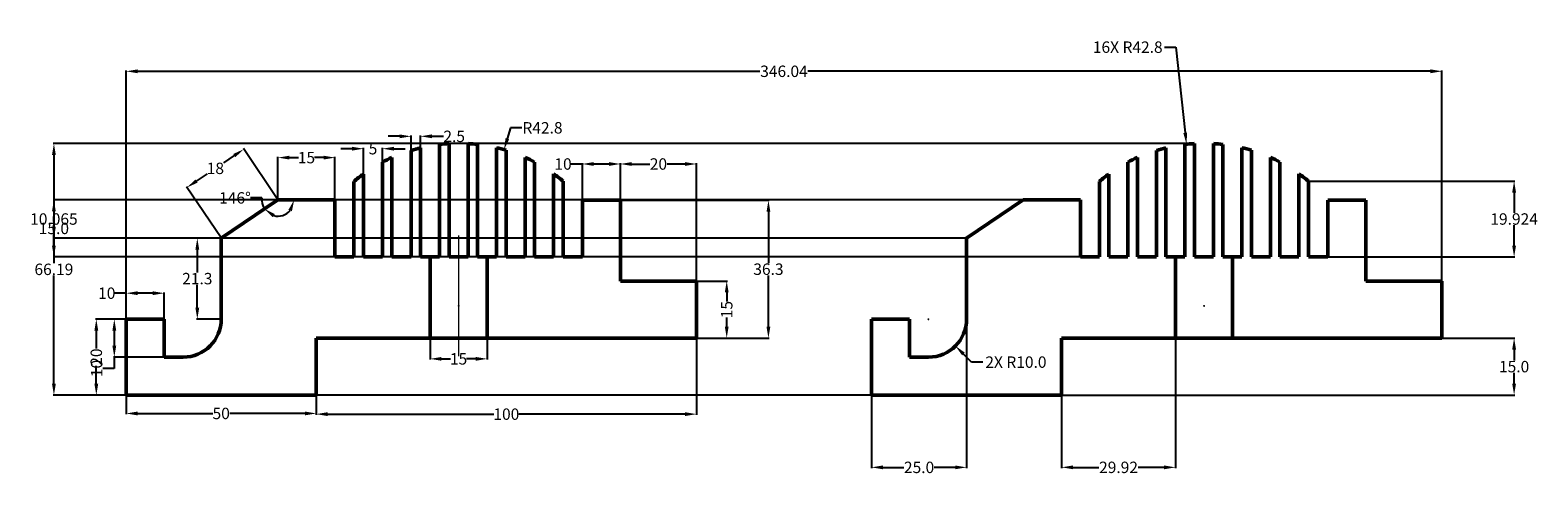
# Model space of a CAD drawing. Units: millimetres. Extents: x 14 to 410, y 16 to 133.
import ezdxf

# ---------------------------------------------------------------- set-up
doc = ezdxf.new("R2010")
doc.units = ezdxf.units.MM
doc.header["$MEASUREMENT"] = 0
doc.linetypes.add('CENTER', pattern=[50.8, 31.75, -6.35, 6.35, -6.35])
for name, color, linetype, lineweight in [('M-CNTR', 7, 'CENTER', 18), ('M-DIMS', 3, 'Continuous', 25), ('M-OUTL', 7, 'Continuous', 50)]:
    doc.layers.add(name, color=color, linetype=linetype, lineweight=lineweight)
doc.styles.get("Standard").update_dxf_attribs({"font": 'arial.ttf'})
doc.dimstyles.get("Standard").update_dxf_attribs({"dimtxt": 3, "dimasz": 3, "dimexe": 0.18, "dimexo": 0.0625, "dimgap": 0.09, "dimtad": 0, "dimtih": 1, "dimtoh": 1, "dimdec": 1, "dimdsep": 46, "dimtxsty": 'Standard', "dimcen": 0.09, "dimadec": 0, "dimazin": 0, "dimtfac": 1, "dimtdec": 1, "dimtofl": 0, "dimtmove": 0, "dimatfit": 3, "dimfxl": 1, "dimtolj": 1, "dimtzin": 0, "dimarcsym": 0})

# ---------------------------------------------------------------- blocks, each defined once
blk = doc.blocks.new('*D1')
at = {"layer": 'Defpoints', "color": 0, "transparency": 16777216}
for p in [(78.96, 88.22), (78.96, 88.22), (93.96, 88.22), (81.78, 85.01), (64.03, 78.16)]:
    blk.add_point(p, dxfattribs=at)
at = {"layer": 'M-DIMS', "color": 0, "lineweight": -2, "transparency": 16777216}
blk.add_line((74.72, 88.75), (71.72, 88.75), dxfattribs=at)
for start, end in [(172.8959, 214), (255.1041, 318.8959)]:
    blk.add_arc((78.96, 88.22), 4.27, start, end, dxfattribs=at)
at = {"layer": 'M-DIMS', "color": 0, "transparency": 16777216}
for points in [[(81.71, 85.59), (82.64, 85.24), (83.23, 88.22)], [(77.57, 83.69), (78.15, 84.5), (75.41, 85.83)]]:
    blk.add_solid(points, dxfattribs=at)
at = {"layer": 'M-DIMS', "color": 0, "transparency": 16777216, "insert": (67.66, 88.75), "char_height": 3, "attachment_point": 5}
blk.add_mtext('\\A1;146°', dxfattribs=at)
blk = doc.blocks.new('*D2')
at = {"layer": 'Defpoints', "color": 0, "transparency": 16777216}
for p in [(169.03, 88.12), (207.96, 88.12), (189.03, 51.86)]:
    blk.add_point(p, dxfattribs=at)
at = {"layer": 'M-DIMS', "color": 0, "lineweight": -2, "transparency": 16777216}
for p, q in [((169.1, 88.12), (208.14, 88.12)), ((207.96, 85.12), (207.96, 71.61)), ((207.96, 54.86), (207.96, 68.37)), ((189.1, 51.86), (208.14, 51.86))]:
    blk.add_line(p, q, dxfattribs=at)
at = {"layer": 'M-DIMS', "color": 0, "transparency": 16777216}
for points in [[(207.46, 85.12), (208.46, 85.12), (207.96, 88.12)], [(207.46, 54.86), (208.46, 54.86), (207.96, 51.86)]]:
    blk.add_solid(points, dxfattribs=at)
at = {"layer": 'M-DIMS', "color": 0, "transparency": 16777216, "insert": (207.96, 69.99), "char_height": 3, "attachment_point": 5}
blk.add_mtext('\\A1;36.3', dxfattribs=at)
blk = doc.blocks.new('*D3')
at = {"layer": 'Defpoints', "color": 0, "transparency": 16777216}
for p in [(189.03, 66.86), (189.03, 51.86), (196.99, 51.86)]:
    blk.add_point(p, dxfattribs=at)
at = {"layer": 'M-DIMS', "color": 0, "lineweight": -2, "transparency": 16777216}
for p, q in [((189.1, 66.86), (197.17, 66.86)), ((196.99, 63.86), (196.99, 61.47)), ((196.99, 54.86), (196.99, 57.25)), ((189.1, 51.86), (197.17, 51.86))]:
    blk.add_line(p, q, dxfattribs=at)
at = {"layer": 'M-DIMS', "color": 0, "transparency": 16777216}
for points in [[(196.49, 63.86), (197.49, 63.86), (196.99, 66.86)], [(196.49, 54.86), (197.49, 54.86), (196.99, 51.86)]]:
    blk.add_solid(points, dxfattribs=at)
at = {"layer": 'M-DIMS', "color": 0, "transparency": 16777216, "insert": (196.99, 59.36), "char_height": 3, "attachment_point": 5, "rotation": 90}
blk.add_mtext('\\A1;15', dxfattribs=at)
blk = doc.blocks.new('*D4')
at = {"layer": 'Defpoints', "color": 0, "transparency": 16777216}
for p in [(159.03, 97.66), (159.03, 88.12), (169.03, 88.12)]:
    blk.add_point(p, dxfattribs=at)
at = {"layer": 'M-DIMS', "color": 0, "lineweight": -2, "transparency": 16777216}
for p, q in [((159.03, 97.66), (156.03, 97.66)), ((159.03, 88.19), (159.03, 97.84)), ((166.03, 97.66), (162.03, 97.66)), ((169.03, 88.19), (169.03, 97.84))]:
    blk.add_line(p, q, dxfattribs=at)
at = {"layer": 'M-DIMS', "color": 0, "transparency": 16777216}
for points in [[(162.03, 98.16), (162.03, 97.16), (159.03, 97.66)], [(166.03, 98.16), (166.03, 97.16), (169.03, 97.66)]]:
    blk.add_solid(points, dxfattribs=at)
at = {"layer": 'M-DIMS', "color": 0, "transparency": 16777216, "insert": (153.94, 97.66), "char_height": 3, "attachment_point": 5}
blk.add_mtext('\\A1;10', dxfattribs=at)
blk = doc.blocks.new('*D5')
at = {"layer": 'Defpoints', "color": 0, "transparency": 16777216}
for p in [(189.03, 97.66), (169.03, 66.86), (189.03, 66.86)]:
    blk.add_point(p, dxfattribs=at)
at = {"layer": 'M-DIMS', "color": 0, "lineweight": -2, "transparency": 16777216}
for p, q in [((169.03, 66.92), (169.03, 97.84)), ((172.03, 97.66), (176.77, 97.66)), ((186.03, 97.66), (181.29, 97.66)), ((189.03, 66.92), (189.03, 97.84))]:
    blk.add_line(p, q, dxfattribs=at)
at = {"layer": 'M-DIMS', "color": 0, "transparency": 16777216}
for points in [[(172.03, 98.16), (172.03, 97.16), (169.03, 97.66)], [(186.03, 98.16), (186.03, 97.16), (189.03, 97.66)]]:
    blk.add_solid(points, dxfattribs=at)
at = {"layer": 'M-DIMS', "color": 0, "transparency": 16777216, "insert": (179.03, 97.66), "char_height": 3, "attachment_point": 5}
blk.add_mtext('\\A1;20', dxfattribs=at)
blk = doc.blocks.new('*D6')
at = {"layer": 'Defpoints', "color": 0, "transparency": 16777216}
for p in [(93.96, 99.34), (78.96, 88.22), (93.96, 88.22)]:
    blk.add_point(p, dxfattribs=at)
at = {"layer": 'M-DIMS', "color": 0, "lineweight": -2, "transparency": 16777216}
for p, q in [((78.96, 88.29), (78.96, 99.52)), ((81.96, 99.34), (84.35, 99.34)), ((90.96, 99.34), (88.56, 99.34)), ((93.96, 88.29), (93.96, 99.52))]:
    blk.add_line(p, q, dxfattribs=at)
at = {"layer": 'M-DIMS', "color": 0, "transparency": 16777216}
for points in [[(81.96, 99.84), (81.96, 98.84), (78.96, 99.34)], [(90.96, 99.84), (90.96, 98.84), (93.96, 99.34)]]:
    blk.add_solid(points, dxfattribs=at)
at = {"layer": 'M-DIMS', "color": 0, "transparency": 16777216, "insert": (86.46, 99.34), "char_height": 3, "attachment_point": 5}
blk.add_mtext('\\A1;15', dxfattribs=at)
blk = doc.blocks.new('*D7')
at = {"layer": 'Defpoints', "color": 0, "transparency": 16777216}
for p in [(69.97, 101.55), (78.96, 88.22), (64.03, 78.16)]:
    blk.add_point(p, dxfattribs=at)
at = {"layer": 'M-DIMS', "color": 0, "lineweight": -2, "transparency": 16777216}
for p, q in [((67.48, 99.87), (64.6, 97.94)), ((78.92, 88.27), (69.86, 101.7)), ((64, 78.21), (54.94, 91.64)), ((57.53, 93.16), (60.4, 95.1))]:
    blk.add_line(p, q, dxfattribs=at)
at = {"layer": 'M-DIMS', "color": 0, "transparency": 16777216}
for points in [[(67.2, 100.29), (67.76, 99.46), (69.97, 101.55)], [(57.25, 93.58), (57.81, 92.75), (55.04, 91.49)]]:
    blk.add_solid(points, dxfattribs=at)
at = {"layer": 'M-DIMS', "color": 0, "transparency": 16777216, "insert": (62.5, 96.52), "char_height": 3, "attachment_point": 5}
blk.add_mtext('\\A1;18', dxfattribs=at)
blk = doc.blocks.new('*D8')
at = {"layer": 'Defpoints', "color": 0, "transparency": 16777216}
for p in [(64.03, 78.16), (57.75, 56.86), (64.03, 56.86)]:
    blk.add_point(p, dxfattribs=at)
at = {"layer": 'M-DIMS', "color": 0, "lineweight": -2, "transparency": 16777216}
for p, q in [((63.97, 78.16), (57.57, 78.16)), ((57.75, 75.16), (57.75, 69.13)), ((57.75, 59.86), (57.75, 65.88)), ((63.97, 56.86), (57.57, 56.86))]:
    blk.add_line(p, q, dxfattribs=at)
at = {"layer": 'M-DIMS', "color": 0, "transparency": 16777216}
for points in [[(57.25, 75.16), (58.25, 75.16), (57.75, 78.16)], [(57.25, 59.86), (58.25, 59.86), (57.75, 56.86)]]:
    blk.add_solid(points, dxfattribs=at)
at = {"layer": 'M-DIMS', "color": 0, "transparency": 16777216, "insert": (57.75, 67.51), "char_height": 3, "attachment_point": 5}
blk.add_mtext('\\A1;21.3', dxfattribs=at)
blk = doc.blocks.new('*D9')
at = {"layer": 'Defpoints', "color": 0, "transparency": 16777216}
for p in [(39.03, 63.68), (39.03, 56.86), (49.03, 56.86)]:
    blk.add_point(p, dxfattribs=at)
at = {"layer": 'M-DIMS', "color": 0, "lineweight": -2, "transparency": 16777216}
for p, q in [((39.03, 63.68), (36.03, 63.68)), ((39.03, 56.92), (39.03, 63.86)), ((46.03, 63.68), (42.03, 63.68)), ((49.03, 56.92), (49.03, 63.86))]:
    blk.add_line(p, q, dxfattribs=at)
at = {"layer": 'M-DIMS', "color": 0, "transparency": 16777216}
for points in [[(42.03, 64.18), (42.03, 63.18), (39.03, 63.68)], [(46.03, 64.18), (46.03, 63.18), (49.03, 63.68)]]:
    blk.add_solid(points, dxfattribs=at)
at = {"layer": 'M-DIMS', "color": 0, "transparency": 16777216, "insert": (33.94, 63.68), "char_height": 3, "attachment_point": 5}
blk.add_mtext('\\A1;10', dxfattribs=at)
blk = doc.blocks.new('*D10')
at = {"layer": 'Defpoints', "color": 0, "transparency": 16777216}
for p in [(39.03, 56.86), (31.18, 36.86), (39.03, 36.86)]:
    blk.add_point(p, dxfattribs=at)
at = {"layer": 'M-DIMS', "color": 0, "lineweight": -2, "transparency": 16777216}
for p, q in [((38.97, 56.86), (31, 56.86)), ((31.18, 53.86), (31.18, 49.12)), ((31.18, 39.86), (31.18, 44.6)), ((38.97, 36.86), (31, 36.86))]:
    blk.add_line(p, q, dxfattribs=at)
at = {"layer": 'M-DIMS', "color": 0, "transparency": 16777216}
for points in [[(30.68, 53.86), (31.68, 53.86), (31.18, 56.86)], [(30.68, 39.86), (31.68, 39.86), (31.18, 36.86)]]:
    blk.add_solid(points, dxfattribs=at)
at = {"layer": 'M-DIMS', "color": 0, "transparency": 16777216, "insert": (31.18, 46.86), "char_height": 3, "attachment_point": 5, "rotation": 90}
blk.add_mtext('\\A1;20', dxfattribs=at)
blk = doc.blocks.new('*D11')
at = {"layer": 'Defpoints', "color": 0, "transparency": 16777216}
for p in [(49.03, 56.86), (35.92, 46.86), (49.03, 46.86)]:
    blk.add_point(p, dxfattribs=at)
at = {"layer": 'M-DIMS', "color": 0, "lineweight": -2, "transparency": 16777216}
for p, q in [((48.97, 56.86), (35.74, 56.86)), ((35.92, 53.86), (35.92, 49.86)), ((35.92, 43.86), (32.92, 43.86)), ((48.97, 46.86), (35.74, 46.86)), ((35.92, 46.86), (35.92, 43.86))]:
    blk.add_line(p, q, dxfattribs=at)
at = {"layer": 'M-DIMS', "color": 0, "transparency": 16777216}
for points in [[(35.42, 53.86), (36.42, 53.86), (35.92, 56.86)], [(35.42, 49.86), (36.42, 49.86), (35.92, 46.86)]]:
    blk.add_solid(points, dxfattribs=at)
at = {"layer": 'M-DIMS', "color": 0, "transparency": 16777216, "insert": (31.29, 43.86), "char_height": 3, "attachment_point": 5, "rotation": 90}
blk.add_mtext('\\A1;10', dxfattribs=at)
blk = doc.blocks.new('*D12')
at = {"layer": 'Defpoints', "color": 0, "transparency": 16777216}
for p in [(39.03, 36.86), (89.03, 36.86), (89.03, 32.04)]:
    blk.add_point(p, dxfattribs=at)
at = {"layer": 'M-DIMS', "color": 0, "lineweight": -2, "transparency": 16777216}
for p, q in [((39.03, 36.79), (39.03, 31.86)), ((89.03, 36.79), (89.03, 31.86)), ((42.03, 32.04), (61.8, 32.04)), ((86.03, 32.04), (66.27, 32.04))]:
    blk.add_line(p, q, dxfattribs=at)
at = {"layer": 'M-DIMS', "color": 0, "transparency": 16777216}
for points in [[(42.03, 32.54), (42.03, 31.54), (39.03, 32.04)], [(86.03, 32.54), (86.03, 31.54), (89.03, 32.04)]]:
    blk.add_solid(points, dxfattribs=at)
at = {"layer": 'M-DIMS', "color": 0, "transparency": 16777216, "insert": (64.03, 32.04), "char_height": 3, "attachment_point": 5}
blk.add_mtext('\\A1;50', dxfattribs=at)
blk = doc.blocks.new('*D13')
at = {"layer": 'Defpoints', "color": 0, "transparency": 16777216}
for p in [(89.03, 51.86), (189.03, 51.86), (189.03, 31.86)]:
    blk.add_point(p, dxfattribs=at)
at = {"layer": 'M-DIMS', "color": 0, "lineweight": -2, "transparency": 16777216}
for p, q in [((89.03, 51.79), (89.03, 31.68)), ((189.03, 51.79), (189.03, 31.68)), ((92.03, 31.86), (135.78, 31.86)), ((186.03, 31.86), (142.29, 31.86))]:
    blk.add_line(p, q, dxfattribs=at)
at = {"layer": 'M-DIMS', "color": 0, "transparency": 16777216}
for points in [[(92.03, 32.36), (92.03, 31.36), (89.03, 31.86)], [(186.03, 32.36), (186.03, 31.36), (189.03, 31.86)]]:
    blk.add_solid(points, dxfattribs=at)
at = {"layer": 'M-DIMS', "color": 0, "transparency": 16777216, "insert": (139.03, 31.86), "char_height": 3, "attachment_point": 5}
blk.add_mtext('\\A1;100', dxfattribs=at)
blk = doc.blocks.new('*D14')
at = {"layer": 'Defpoints', "color": 0, "transparency": 16777216}
for p in [(138.44, 101.42), (126.49, 60.32)]:
    blk.add_point(p, dxfattribs=at)
at = {"layer": 'M-DIMS', "color": 0, "lineweight": -2, "transparency": 16777216}
for p, q in [((140.12, 107.18), (139.28, 104.3)), ((143.12, 107.18), (140.12, 107.18)), ((126.4, 60.32), (126.58, 60.32)), ((126.49, 60.23), (126.49, 60.41))]:
    blk.add_line(p, q, dxfattribs=at)
at = {"layer": 'M-DIMS', "color": 0, "transparency": 16777216}
blk.add_solid([(138.8, 104.44), (139.76, 104.16), (138.44, 101.42)], dxfattribs=at)
at = {"layer": 'M-DIMS', "color": 0, "transparency": 16777216, "insert": (148.54, 107.18), "char_height": 3, "attachment_point": 5}
blk.add_mtext('\\A1;R42.8', dxfattribs=at)
blk = doc.blocks.new('*D15')
at = {"layer": 'Defpoints', "color": 0, "transparency": 16777216}
for p in [(116.46, 104.94), (113.96, 101.24), (116.46, 101.92)]:
    blk.add_point(p, dxfattribs=at)
at = {"layer": 'M-DIMS', "color": 0, "lineweight": -2, "transparency": 16777216}
for p, q in [((110.96, 104.94), (107.96, 104.94)), ((113.96, 101.3), (113.96, 105.12)), ((116.46, 101.99), (116.46, 105.12)), ((119.46, 104.94), (122.46, 104.94))]:
    blk.add_line(p, q, dxfattribs=at)
at = {"layer": 'M-DIMS', "color": 0, "transparency": 16777216}
for points in [[(110.96, 105.44), (110.96, 104.44), (113.96, 104.94)], [(119.46, 105.44), (119.46, 104.44), (116.46, 104.94)]]:
    blk.add_solid(points, dxfattribs=at)
at = {"layer": 'M-DIMS', "color": 0, "transparency": 16777216, "insert": (125.31, 104.94), "char_height": 3, "attachment_point": 5}
blk.add_mtext('\\A1;2.5', dxfattribs=at)
blk = doc.blocks.new('*D16')
at = {"layer": 'Defpoints', "color": 0, "transparency": 16777216}
for p in [(106.46, 101.69), (101.46, 95.03), (106.46, 95.03)]:
    blk.add_point(p, dxfattribs=at)
at = {"layer": 'M-DIMS', "color": 0, "lineweight": -2, "transparency": 16777216}
for p, q in [((98.46, 101.69), (95.46, 101.69)), ((101.46, 95.09), (101.46, 101.87)), ((106.46, 95.09), (106.46, 101.87)), ((109.46, 101.69), (112.46, 101.69))]:
    blk.add_line(p, q, dxfattribs=at)
at = {"layer": 'M-DIMS', "color": 0, "transparency": 16777216}
for points in [[(98.46, 102.19), (98.46, 101.19), (101.46, 101.69)], [(109.46, 102.19), (109.46, 101.19), (106.46, 101.69)]]:
    blk.add_solid(points, dxfattribs=at)
at = {"layer": 'M-DIMS', "color": 0, "transparency": 16777216, "insert": (103.96, 101.69), "char_height": 3, "attachment_point": 5}
blk.add_mtext('\\A1;5', dxfattribs=at)
blk = doc.blocks.new('*D17')
at = {"layer": 'Defpoints', "color": 0, "transparency": 16777216}
for p in [(118.96, 51.86), (133.96, 51.86), (133.96, 46.4)]:
    blk.add_point(p, dxfattribs=at)
at = {"layer": 'M-DIMS', "color": 0, "lineweight": -2, "transparency": 16777216}
for p, q in [((118.96, 51.79), (118.96, 46.22)), ((133.96, 51.79), (133.96, 46.22)), ((121.96, 46.4), (124.35, 46.4)), ((130.96, 46.4), (128.56, 46.4))]:
    blk.add_line(p, q, dxfattribs=at)
at = {"layer": 'M-DIMS', "color": 0, "transparency": 16777216}
for points in [[(121.96, 46.9), (121.96, 45.9), (118.96, 46.4)], [(130.96, 46.9), (130.96, 45.9), (133.96, 46.4)]]:
    blk.add_solid(points, dxfattribs=at)
at = {"layer": 'M-DIMS', "color": 0, "transparency": 16777216, "insert": (126.46, 46.4), "char_height": 3, "attachment_point": 5}
blk.add_mtext('\\A1;15', dxfattribs=at)
blk = doc.blocks.new('HEAT-SINK-PROFILE-150')
for p, q in [((74.92, 36.37), (74.92, 64.38)), ((77.42, 36.37), (77.42, 65.07)), ((82.42, 36.37), (82.42, 65.96)), ((84.92, 36.37), (84.92, 66.19)), ((89.92, 36.37), (89.92, 66.19)), ((92.42, 36.37), (92.42, 65.97)), ((97.42, 36.37), (97.42, 65.09)), ((99.92, 36.37), (99.92, 64.41)), ((67.42, 36.37), (67.42, 61.28)), ((69.92, 36.37), (69.92, 62.5)), ((104.92, 36.37), (104.92, 62.54)), ((107.42, 36.37), (107.42, 61.32)), ((59.92, 36.37), (59.92, 56.22)), ((62.42, 36.37), (62.42, 58.17)), ((112.42, 36.37), (112.42, 58.23)), ((114.92, 36.37), (114.92, 56.29)), ((25, 41.3), (39.92, 51.37)), ((39.92, 51.37), (54.92, 51.37)), ((54.92, 36.37), (54.92, 51.37)), ((120, 51.27), (120, 36.37)), ((130, 51.27), (120, 51.27)), ((130, 30), (130, 51.27)), ((25, 20), (25, 41.3)), ((59.92, 36.37), (54.92, 36.37)), ((67.42, 36.37), (62.42, 36.37)), ((74.92, 36.37), (69.92, 36.37)), ((82.42, 36.37), (77.42, 36.37)), ((79.92, 36.37), (79.92, 15)), ((89.92, 36.37), (84.92, 36.37)), ((97.42, 36.37), (92.42, 36.37)), ((94.92, 36.37), (94.92, 15)), ((104.92, 36.37), (99.92, 36.37)), ((112.42, 36.37), (107.42, 36.37)), ((120, 36.37), (114.92, 36.37)), ((150, 30), (130, 30)), ((150, 15), (150, 30)), ((0, 0), (0, 20)), ((0, 20), (10, 20)), ((10, 20), (10, 10)), ((50, 0), (50, 15)), ((50, 15), (150, 15)), ((10, 10), (15, 10)), ((50, 0), (0, 0))]:
    blk.add_line(p, q)
for centre, radius, start, end in [((87.46, 23.46), 42.8, 103.565, 107.0352), ((87.46, 23.46), 42.8, 93.4005, 96.7609), ((87.46, 23.46), 42.8, 83.3434, 86.7032), ((87.46, 23.46), 42.8, 73.073, 76.5415), ((87.46, 23.46), 42.8, 114.1911, 117.9171), ((87.46, 23.46), 42.8, 62.2, 65.9223), ((87.46, 23.46), 42.8, 125.8041, 130.0478), ((87.46, 23.46), 42.8, 50.0873, 54.3234), ((15, 20), 10, 270, 0)]:
    blk.add_arc(centre, radius, start, end)
blk = doc.blocks.new('*D19')
at = {"layer": 'Defpoints', "color": 0, "transparency": 16777216}
for p in [(260.08, 56.86), (235.08, 36.86), (260.08, 17.86)]:
    blk.add_point(p, dxfattribs=at)
at = {"layer": 'M-DIMS', "color": 0, "lineweight": -2, "transparency": 16777216}
for p, q in [((260.08, 56.79), (260.08, 17.68)), ((235.08, 36.79), (235.08, 17.68)), ((238.08, 17.86), (243.57, 17.86)), ((257.08, 17.86), (251.58, 17.86))]:
    blk.add_line(p, q, dxfattribs=at)
at = {"layer": 'M-DIMS', "color": 0, "transparency": 16777216}
for points in [[(238.08, 18.36), (238.08, 17.36), (235.08, 17.86)], [(257.08, 18.36), (257.08, 17.36), (260.08, 17.86)]]:
    blk.add_solid(points, dxfattribs=at)
at = {"layer": 'M-DIMS', "color": 0, "transparency": 16777216, "insert": (247.58, 17.86), "char_height": 3, "attachment_point": 5}
blk.add_mtext('\\A1;25.0', dxfattribs=at)
blk = doc.blocks.new('*D20')
at = {"layer": 'Defpoints', "color": 0, "transparency": 16777216}
for p in [(20.03, 88.22), (275, 88.22), (260.08, 78.16)]:
    blk.add_point(p, dxfattribs=at)
at = {"layer": 'M-DIMS', "color": 0, "lineweight": -2, "transparency": 16777216}
for p, q in [((274.94, 88.22), (19.85, 88.22)), ((20.03, 85.22), (20.03, 84.81)), ((20.03, 81.16), (20.03, 81.57)), ((260.01, 78.16), (19.85, 78.16))]:
    blk.add_line(p, q, dxfattribs=at)
at = {"layer": 'M-DIMS', "color": 0, "transparency": 16777216}
for points in [[(19.53, 85.22), (20.53, 85.22), (20.03, 88.22)], [(19.53, 81.16), (20.53, 81.16), (20.03, 78.16)]]:
    blk.add_solid(points, dxfattribs=at)
at = {"layer": 'M-DIMS', "color": 0, "transparency": 16777216, "insert": (20.03, 83.19), "char_height": 3, "attachment_point": 5}
blk.add_mtext('\\A1;10.065', dxfattribs=at)
blk = doc.blocks.new('*D21')
at = {"layer": 'Defpoints', "color": 0, "transparency": 16777216}
for p in [(290, 88.22), (20.03, 73.22), (290, 73.22)]:
    blk.add_point(p, dxfattribs=at)
at = {"layer": 'M-DIMS', "color": 0, "lineweight": -2, "transparency": 16777216}
for p, q in [((289.94, 88.22), (19.85, 88.22)), ((20.03, 85.22), (20.03, 82.34)), ((20.03, 76.22), (20.03, 79.1)), ((289.94, 73.22), (19.85, 73.22))]:
    blk.add_line(p, q, dxfattribs=at)
at = {"layer": 'M-DIMS', "color": 0, "transparency": 16777216}
for points in [[(19.53, 85.22), (20.53, 85.22), (20.03, 88.22)], [(19.53, 76.22), (20.53, 76.22), (20.03, 73.22)]]:
    blk.add_solid(points, dxfattribs=at)
at = {"layer": 'M-DIMS', "color": 0, "transparency": 16777216, "insert": (20.03, 80.72), "char_height": 3, "attachment_point": 5}
blk.add_mtext('\\A1;15.0', dxfattribs=at)
blk = doc.blocks.new('*D22')
at = {"layer": 'Defpoints', "color": 0, "transparency": 16777216}
for p in [(350, 93.15), (404.08, 93.15), (350, 73.22)]:
    blk.add_point(p, dxfattribs=at)
at = {"layer": 'M-DIMS', "color": 0, "lineweight": -2, "transparency": 16777216}
for p, q in [((350.06, 93.15), (404.26, 93.15)), ((404.08, 90.15), (404.08, 84.81)), ((404.08, 76.22), (404.08, 81.56)), ((350.06, 73.22), (404.26, 73.22))]:
    blk.add_line(p, q, dxfattribs=at)
at = {"layer": 'M-DIMS', "color": 0, "transparency": 16777216}
for points in [[(403.58, 90.15), (404.58, 90.15), (404.08, 93.15)], [(403.58, 76.22), (404.58, 76.22), (404.08, 73.22)]]:
    blk.add_solid(points, dxfattribs=at)
at = {"layer": 'M-DIMS', "color": 0, "transparency": 16777216, "insert": (404.08, 83.19), "char_height": 3, "attachment_point": 5}
blk.add_mtext('\\A1;19.924', dxfattribs=at)
blk = doc.blocks.new('*D23')
at = {"layer": 'Defpoints', "color": 0, "transparency": 16777216}
for p in [(285.08, 51.86), (315, 51.86), (315, 17.86)]:
    blk.add_point(p, dxfattribs=at)
at = {"layer": 'M-DIMS', "color": 0, "lineweight": -2, "transparency": 16777216}
for p, q in [((285.08, 51.79), (285.08, 17.68)), ((315, 51.79), (315, 17.68)), ((288.08, 17.86), (294.87, 17.86)), ((312, 17.86), (305.2, 17.86))]:
    blk.add_line(p, q, dxfattribs=at)
at = {"layer": 'M-DIMS', "color": 0, "transparency": 16777216}
for points in [[(288.08, 18.36), (288.08, 17.36), (285.08, 17.86)], [(312, 18.36), (312, 17.36), (315, 17.86)]]:
    blk.add_solid(points, dxfattribs=at)
at = {"layer": 'M-DIMS', "color": 0, "transparency": 16777216, "insert": (300.04, 17.86), "char_height": 3, "attachment_point": 5}
blk.add_mtext('\\A1;29.92', dxfattribs=at)
blk = doc.blocks.new('*D24')
at = {"layer": 'Defpoints', "color": 0, "transparency": 16777216}
for p in [(385.08, 51.86), (404.08, 51.86), (285.08, 36.86)]:
    blk.add_point(p, dxfattribs=at)
at = {"layer": 'M-DIMS', "color": 0, "lineweight": -2, "transparency": 16777216}
for p, q in [((385.14, 51.86), (404.26, 51.86)), ((404.08, 48.86), (404.08, 45.98)), ((404.08, 39.86), (404.08, 42.74)), ((285.14, 36.86), (404.26, 36.86))]:
    blk.add_line(p, q, dxfattribs=at)
at = {"layer": 'M-DIMS', "color": 0, "transparency": 16777216}
for points in [[(403.58, 48.86), (404.58, 48.86), (404.08, 51.86)], [(403.58, 39.86), (404.58, 39.86), (404.08, 36.86)]]:
    blk.add_solid(points, dxfattribs=at)
at = {"layer": 'M-DIMS', "color": 0, "transparency": 16777216, "insert": (404.08, 44.36), "char_height": 3, "attachment_point": 5}
blk.add_mtext('\\A1;15.0', dxfattribs=at)
blk = doc.blocks.new('*D25')
at = {"layer": 'Defpoints', "color": 0, "transparency": 16777216}
for p in [(20.03, 103.04), (320, 103.04), (235.08, 36.86)]:
    blk.add_point(p, dxfattribs=at)
at = {"layer": 'M-DIMS', "color": 0, "lineweight": -2, "transparency": 16777216}
for p, q in [((319.94, 103.04), (19.85, 103.04)), ((20.03, 100.04), (20.03, 71.57)), ((20.03, 39.86), (20.03, 68.33)), ((235.01, 36.86), (19.85, 36.86))]:
    blk.add_line(p, q, dxfattribs=at)
at = {"layer": 'M-DIMS', "color": 0, "transparency": 16777216}
for points in [[(19.53, 100.04), (20.53, 100.04), (20.03, 103.04)], [(19.53, 39.86), (20.53, 39.86), (20.03, 36.86)]]:
    blk.add_solid(points, dxfattribs=at)
at = {"layer": 'M-DIMS', "color": 0, "transparency": 16777216, "insert": (20.03, 69.95), "char_height": 3, "attachment_point": 5}
blk.add_mtext('\\A1;66.19', dxfattribs=at)
blk = doc.blocks.new('*D26')
at = {"layer": 'Defpoints', "color": 0, "transparency": 16777216}
for p in [(385.08, 122.05), (385.08, 66.86), (39.03, 56.86)]:
    blk.add_point(p, dxfattribs=at)
at = {"layer": 'M-DIMS', "color": 0, "lineweight": -2, "transparency": 16777216}
for p, q in [((39.03, 56.92), (39.03, 122.23)), ((42.03, 122.05), (205.74, 122.05)), ((382.08, 122.05), (218.36, 122.05)), ((385.08, 66.92), (385.08, 122.23))]:
    blk.add_line(p, q, dxfattribs=at)
at = {"layer": 'M-DIMS', "color": 0, "transparency": 16777216}
for points in [[(42.03, 122.55), (42.03, 121.55), (39.03, 122.05)], [(382.08, 122.55), (382.08, 121.55), (385.08, 122.05)]]:
    blk.add_solid(points, dxfattribs=at)
at = {"layer": 'M-DIMS', "color": 0, "transparency": 16777216, "insert": (212.05, 122.05), "char_height": 3, "attachment_point": 5}
blk.add_mtext('\\A1;346.04', dxfattribs=at)
blk = doc.blocks.new('*D27')
at = {"layer": 'Defpoints', "color": 0, "transparency": 16777216}
for p in [(317.91, 102.87), (322.54, 60.32)]:
    blk.add_point(p, dxfattribs=at)
at = {"layer": 'M-DIMS', "color": 0, "lineweight": -2, "transparency": 16777216}
for p, q in [((312.13, 128.4), (315.13, 128.4)), ((315.13, 128.4), (317.58, 105.85)), ((322.45, 60.32), (322.63, 60.32)), ((322.54, 60.23), (322.54, 60.41))]:
    blk.add_line(p, q, dxfattribs=at)
at = {"layer": 'M-DIMS', "color": 0, "transparency": 16777216}
blk.add_solid([(318.08, 105.9), (317.09, 105.8), (317.91, 102.87)], dxfattribs=at)
at = {"layer": 'M-DIMS', "color": 0, "transparency": 16777216, "insert": (302.46, 128.4), "char_height": 3, "attachment_point": 5}
blk.add_mtext('\\A1;16X R42.8', dxfattribs=at)
blk = doc.blocks.new('*D28')
at = {"layer": 'Defpoints', "color": 0, "transparency": 16777216}
for p in [(250.08, 56.86), (257.15, 49.79)]:
    blk.add_point(p, dxfattribs=at)
at = {"layer": 'M-DIMS', "color": 0, "lineweight": -2, "transparency": 16777216}
for p, q in [((249.99, 56.86), (250.17, 56.86)), ((250.08, 56.77), (250.08, 56.95)), ((261.39, 45.54), (259.27, 47.66)), ((264.39, 45.54), (261.39, 45.54))]:
    blk.add_line(p, q, dxfattribs=at)
at = {"layer": 'M-DIMS', "color": 0, "transparency": 16777216}
blk.add_solid([(259.62, 48.02), (258.91, 47.31), (257.15, 49.79)], dxfattribs=at)
at = {"layer": 'M-DIMS', "color": 0, "transparency": 16777216, "insert": (273.05, 45.54), "char_height": 3, "attachment_point": 5}
blk.add_mtext('\\A1;2X R10.0', dxfattribs=at)

msp = doc.modelspace()

# ---------------------------------------------------------------- linework, layer by layer
at = {"layer": 'M-CNTR'}
msp.add_line((126.4555, 78.884), (126.4555, 45.5699), dxfattribs=at)

# ---------------------------------------------------------------- block references
at = {"layer": 'M-OUTL'}
for p in [(39.0329, 36.8574), (235.0754, 36.8574)]:
    msp.add_blockref('HEAT-SINK-PROFILE-150', p, dxfattribs=at)

# ---------------------------------------------------------------- dimensions: what is measured, and where the dimension line sits
at = {"layer": 'M-DIMS'}
for center, mpoint, text, picture, middle in [((322.5368, 60.3186), (317.909, 102.8677), '16X <>', '*D27', (302.4601, 128.3971)), ((250.0754, 56.8574), (257.1461, 49.7859), '2X <>', '*D28', (273.0539, 45.543))]:
    dim = msp.add_radius_dim(center=center, mpoint=mpoint, text=text, dimstyle='Standard', override={"dimdec": 1, "dimlfac": 1, "dimrnd": 0, "dimzin": 0, "dimdsep": 46, "dimlunit": 2}, dxfattribs=at)
    dim.commit()
    dim.dimension.update_dxf_attribs({"geometry": picture, "text_midpoint": middle, "dimtype": 164})
for base, p1, p2, override, picture, middle in [((385.0754, 122.0478), (39.0329, 56.8574), (385.0754, 66.8574), {"dimdec": 2, "dimlfac": 1, "dimrnd": 0, "dimzin": 0, "dimdsep": 46, "dimlunit": 2}, '*D26', (212.0541, 122.0478)), ((260.0754, 17.8574), (235.0754, 36.8574), (260.0754, 56.8574), {"dimdec": 1, "dimlfac": 1, "dimrnd": 0, "dimzin": 0, "dimdsep": 46, "dimlunit": 2}, '*D19', (247.5754, 17.8574)), ((314.9981, 17.8574), (285.0754, 51.8574), (314.9981, 51.8574), {"dimdec": 2, "dimlfac": 1, "dimrnd": 0, "dimzin": 0, "dimdsep": 46, "dimlunit": 2}, '*D23', (300.0368, 17.8574))]:
    dim = msp.add_linear_dim(base=base, p1=p1, p2=p2, dimstyle='Standard', override=override, dxfattribs=at)
    dim.commit()
    dim.dimension.update_dxf_attribs({"geometry": picture, "text_midpoint": middle})
at = {"layer": 'M-DIMS', "transparency": 33554610}
dim = msp.add_radius_dim(center=(126.4942, 60.3186), mpoint=(138.441, 101.4174), dimstyle='Standard', override={"dimclrd": 0, "dimclre": 0, "dimclrt": 0}, dxfattribs=at)
dim.commit()
dim.dimension.update_dxf_attribs({"geometry": '*D14', "text_midpoint": (148.5407, 107.179)})
for base, p1, p2, picture, middle in [((106.4555, 101.6933), (101.4555, 95.0304), (106.4555, 95.0304), '*D16', (103.9555, 101.6933)), ((116.4555, 104.9372), (113.9555, 101.2408), (116.4555, 101.9247), '*D15', (125.3133, 104.9372)), ((93.9555, 99.3352), (78.9555, 88.2228), (93.9555, 88.2228), '*D6', (86.4555, 99.3352)), ((159.0329, 97.6582), (169.0329, 88.1228), (159.0329, 88.1228), '*D4', (153.9405, 97.6582)), ((189.0329, 97.6582), (169.0329, 66.8574), (189.0329, 66.8574), '*D5', (179.0329, 97.6582)), ((39.0329, 63.6839), (49.0329, 56.8574), (39.0329, 56.8574), '*D9', (33.9405, 63.6839)), ((189.0329, 31.8614), (89.0329, 51.8574), (189.0329, 51.8574), '*D13', (139.0329, 31.8614)), ((133.9555, 46.4032), (118.9555, 51.8574), (133.9555, 51.8574), '*D17', (126.4555, 46.4032)), ((89.0329, 32.0414), (39.0329, 36.8574), (89.0329, 36.8574), '*D12', (64.0329, 32.0414))]:
    dim = msp.add_linear_dim(base=base, p1=p1, p2=p2, dimstyle='Standard', override={"dimclrd": 0, "dimclre": 0, "dimclrt": 0}, dxfattribs=at)
    dim.commit()
    dim.dimension.update_dxf_attribs({"geometry": picture, "text_midpoint": middle})
at = {"layer": 'M-DIMS'}
for base, p1, p2, override, picture, middle in [((20.0329, 103.0433), (235.0754, 36.8574), (319.9981, 103.0433), {"dimdec": 2, "dimlfac": 1, "dimrnd": 0, "dimzin": 0, "dimdsep": 46, "dimlunit": 2}, '*D25', (20.0329, 69.9503)), ((404.0754, 93.1472), (349.9981, 73.2228), (349.9981, 93.1472), {"dimdec": 3, "dimlfac": 1, "dimrnd": 0, "dimzin": 0, "dimdsep": 46, "dimlunit": 2}, '*D22', (404.0754, 83.185)), ((20.0329, 88.2228), (260.0754, 78.1574), (274.9981, 88.2228), {"dimdec": 3, "dimlfac": 1, "dimrnd": 0, "dimzin": 0, "dimdsep": 46, "dimlunit": 2}, '*D20', (20.0329, 83.1901)), ((20.0329, 73.2228), (289.9981, 88.2228), (289.9981, 73.2228), {"dimdec": 1, "dimlfac": 1, "dimrnd": 0, "dimzin": 0, "dimdsep": 46, "dimlunit": 2}, '*D21', (20.0329, 80.7228)), ((404.0754, 51.8574), (285.0754, 36.8574), (385.0754, 51.8574), {"dimdec": 1, "dimlfac": 1, "dimrnd": 0, "dimzin": 0, "dimdsep": 46, "dimlunit": 2}, '*D24', (404.0754, 44.3574))]:
    dim = msp.add_linear_dim(base=base, p1=p1, p2=p2, angle=90, dimstyle='Standard', override=override, dxfattribs=at)
    dim.commit()
    dim.dimension.update_dxf_attribs({"geometry": picture, "text_midpoint": middle})
at = {"layer": 'M-DIMS', "transparency": 33554610}
dim = msp.add_aligned_dim(p1=(64.0329, 78.1574), p2=(78.9555, 88.2228), distance=16.0774, dimstyle='Standard', override={"dimclrd": 0, "dimclre": 0, "dimclrt": 0}, dxfattribs=at)
dim.commit()
dim.dimension.update_dxf_attribs({"geometry": '*D7', "text_midpoint": (62.5039, 96.5189)})
dim = msp.add_angular_dim_2l(base=(81.7775, 85.0145), line1=((78.9555, 88.2228), (93.9555, 88.2228)), line2=((64.0329, 78.1574), (78.9555, 88.2228)), dimstyle='Standard', override={"dimclrd": 0, "dimclre": 0, "dimclrt": 0}, dxfattribs=at)
dim.commit()
dim.dimension.update_dxf_attribs({"geometry": '*D1', "text_midpoint": (67.6586, 88.7513)})
for base, p1, p2, picture, middle in [((207.9584, 88.1228), (189.0329, 51.8574), (169.0329, 88.1228), '*D2', (207.9584, 69.9901)), ((57.7475, 56.8574), (64.0329, 78.1574), (64.0329, 56.8574), '*D8', (57.7475, 67.5074))]:
    dim = msp.add_linear_dim(base=base, p1=p1, p2=p2, angle=90, dimstyle='Standard', override={"dimclrd": 0, "dimclre": 0, "dimclrt": 0}, dxfattribs=at)
    dim.commit()
    dim.dimension.update_dxf_attribs({"geometry": picture, "text_midpoint": middle})
for base, p1, p2, picture, middle in [((196.9907, 51.8574), (189.0329, 66.8574), (189.0329, 51.8574), '*D3', (196.9907, 59.3574)), ((31.1792, 36.8574), (39.0329, 56.8574), (39.0329, 36.8574), '*D10', (31.1792, 46.8574)), ((35.9157, 46.8574), (49.0329, 56.8574), (49.0329, 46.8574), '*D11', (31.294, 43.8574))]:
    dim = msp.add_linear_dim(base=base, p1=p1, p2=p2, angle=90, dimstyle='Standard', override={"dimclrd": 0, "dimclre": 0, "dimclrt": 0}, dxfattribs=at)
    dim.commit()
    dim.dimension.update_dxf_attribs({"geometry": picture, "text_midpoint": middle, "text_rotation": 90})

doc.saveas('drawing.dxf')
